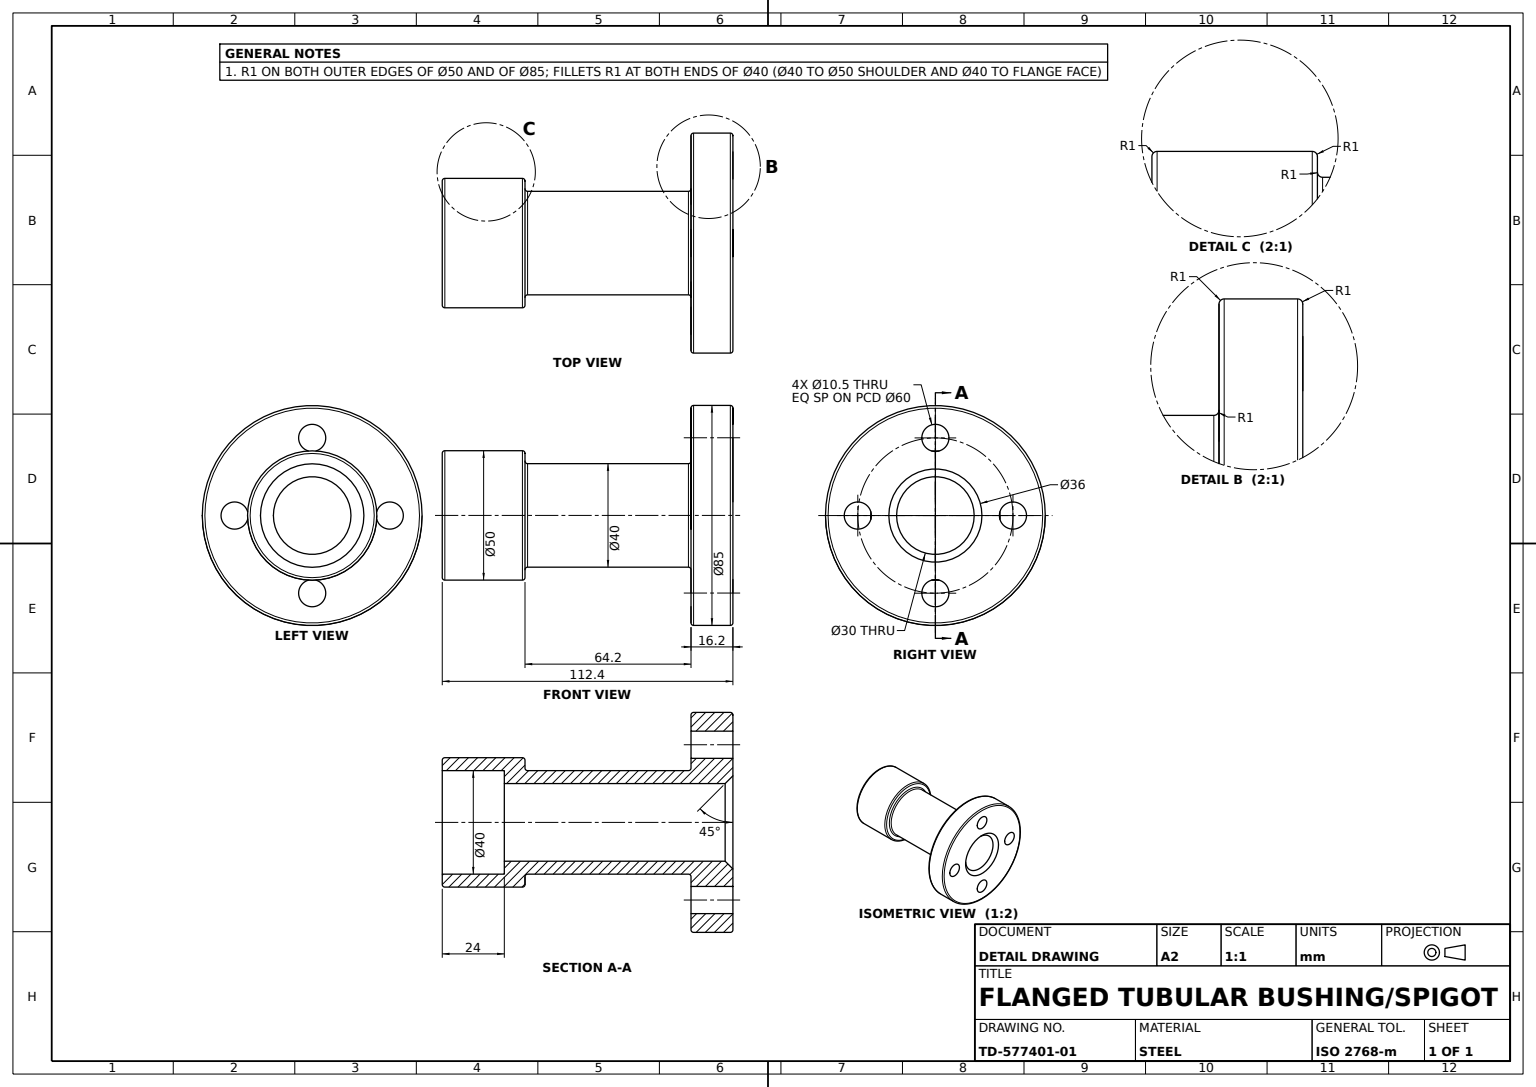
SolidWorks part; units mm, degrees
material "Plain Carbon Steel"
ref_plane "Front Plane" through (0, 0, 0) normal (0, 0, 1) x (1, 0, 0)
ref_plane "Top Plane" through (0, 0, 0) normal (0, 1, 0) x (1, 0, 0)
ref_plane "Right Plane" through (0, 0, 0) normal (1, 0, 0) x (0, 0, -1)
sketch "Bush Profile Sketch" plane through (0, 0, 0) normal (1, 0, 0) x (0, 0, -1)
  line L0 (-511.4646, 0) -> (25061.7632, 0) construction
  line L1 (0, -511.4646) -> (0, 25061.7632) construction
  line L2 (0, 15) -> (0, 42.5)
  line L3 (0, 42.5) -> (-16.2, 42.5)
  line L4 (-16.2, 42.5) -> (-16.2, 20)
  line L5 (-16.2, 20) -> (-80.4, 20)
  line L6 (-80.4, 20) -> (-80.4, 25)
  line L7 (-80.4, 25) -> (-112.4, 25)
  line L8 (-112.4, 25) -> (-112.4, 20)
  line L9 (-112.4, 20) -> (-88.4, 20)
  line L10 (-88.4, 20) -> (-88.4, 15)
  line L11 (-88.4, 15) -> (0, 15)
  dimension "D1" = 42.5
  dimension "D2" = 15
  dimension "D3" = 20
  dimension "D4" = 16.2
  dimension "D5" = 24
  dimension "D6" = 8
  dimension "D7" = 64.2
  dimension "D8" = 20
  dimension "D9" = 25
revolve "Flanged Bush Body" add sketch "Bush Profile Sketch" angle 360 about L0
sketch "Flange Holes Sketch" plane through (0, 0, 0) normal (0, 0, -1) x (-1, 0, 0)
  line L0 (-1000, 0) -> (49000, 0) construction
  line L1 (0, -1000) -> (0, 49000) construction
  circle A0 centre (0, 0) radius 30 construction
  circle A1 centre (0, 30) radius 5.25
  circle A2 centre (30, 0) radius 5.25
  circle A3 centre (0, -30) radius 5.25
  circle A4 centre (-30, 0) radius 5.25
  point P18 (0, 0)
  dimension "D1" = 60
  dimension "D2" = 10.5
  dimension "D3" = 4
extrude "Flange Holes 4xØ10.5" cut sketch "Flange Holes Sketch" against normal blind 39
chamfer "Chamfer 3x45" distance 3 angle 45 1 edges at (15, 0, 0)
fillet "Fillet R1" radius 1 6 edges at (20, 0, 80.4) (25, 0, 112.4) (25, 0, 80.4) (20, 0, 16.2) (42.5, 0, 16.2) (42.5, 0, 0)
